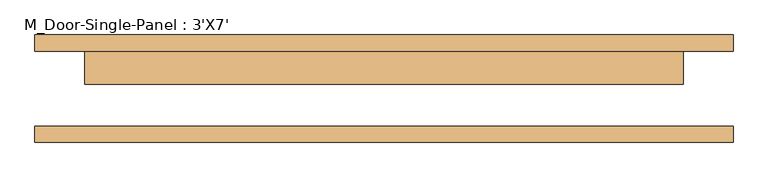
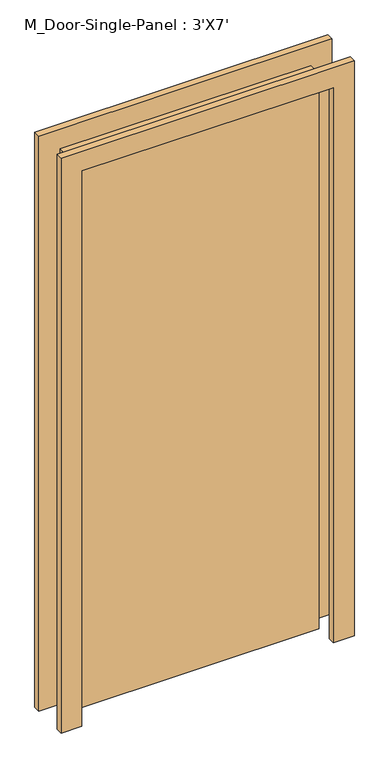
"""IFC4 building model written with IfcOpenShell, lengths in millimetres: door geometry, M_Door-Single-Panel : 3'X7'."""

from ifc_helpers import new_model, si_unit, frame, origin, origin_with_axes, place, context, project, spatial, polyline, outline, extrude, source, transform, mapped, element, save


def m_door_single_panel_3_x7_f8176753(model_context):
    return source(origin(), model_context, "Body", "SweptSolid", [
        extrude(outline(polyline([(457.2, 7.15), (-457.2, 7.15), (-457.2, 57.15), (457.2, 57.15), (457.2, 7.15)])), origin_with_axes(), (0.0, 0.0, 1.0), 2133.6),
        extrude(outline(polyline([(2209.8, 533.4), (2209.8, -533.4), (0.0, -533.4), (0.0, -457.2), (2133.6, -457.2), (2133.6, 457.2), (0.0, 457.2), (0.0, 533.4), (2209.8, 533.4)])), frame((0.0, -82.15, 0.0), z_axis=(0.0, 1.0, 0.0), x_axis=(0.0, 0.0, 1.0)), (0.0, 0.0, 1.0), 25.0),
        extrude(outline(polyline([(2209.8, -533.4), (0.0, -533.4), (0.0, -457.2), (2133.6, -457.2), (2133.6, 457.2), (0.0, 457.2), (0.0, 533.4), (2209.8, 533.4), (2209.8, -533.4)])), frame((0.0, 57.15, 0.0), z_axis=(0.0, 1.0, 0.0), x_axis=(0.0, 0.0, 1.0)), (0.0, 0.0, 1.0), 25.0),
    ])


if __name__ == "__main__":
    model = new_model("IFC4")
    model_context = context("Model", 3, world=origin())
    ifc_project = project(units=[si_unit("LENGTHUNIT", "METRE", prefix="MILLI")], contexts=[model_context])
    site = spatial("IfcSite", under=ifc_project)
    building = spatial("IfcBuilding", under=site)
    placement = place(None, origin())
    m_door_single_panel_3_x7_shape = m_door_single_panel_3_x7_f8176753(model_context)
    element("IfcDoor", 1, ObjectType="M_Door-Single-Panel : 3'X7'", at=placement, inside=building, context=model_context, shape_type="MappedRepresentation", body=[
        mapped(m_door_single_panel_3_x7_shape, transform((0.0, 0.0, 0.0), x_axis=(1.0, 0.0, 0.0), y_axis=(0.0, 1.0, 0.0), z_axis=(0.0, 0.0, 1.0))),
    ])
    save(model, "model.ifc")

# Revit data of these elements
# Type "M_Door-Single-Panel : 3'X7'"
#   Type Mark = "11"
#   Construction Type Id = "DOOR"
#   Assembly Code = "C1020300"
#   Analytic Construction = "Wooden"
#   Thickness = 0' - 1.9685"
#   Thermal Resistance (R) = 2.5876 (h·ft²·°F)/BTU
#   Swing Angle [instance default] = 90.00°
#   Heat Transfer Coefficient (U) = 0.3865 BTU/(h·ft²·°F)
#   Height = 7' - 0"
#   Trim Projection Ext = 0' - 0.98425"
#   Trim Projection Int = 0' - 0.98425"
#   Trim Width = 0' - 3.14961"
#   Width = 3' - 0"
#   Define Thermal Properties by = 1
#   Panel Material = Wood - Birch - Solid Stained Light Low Gloss
#   Trim Material = Paint - Sienna
#   Visual Light Transmittance = 0
#   Solar Heat Gain Coefficient = 0
#   Function = (empty or 0)
#   Wall Closure = (empty or 0)
# Element 1 (IfcDoor, "M_Door-Single-Panel : 3'X7'")
#   Materials on its faces: "Paint - Sienna", "Wood - Birch - Solid Stained Light Low Gloss"
# Materials
#   "Wood - Birch - Solid Stained Light Low Gloss": class "Wood", colour RGB 210 159 95, transparency 0, Cost = 0
#   "Paint - Sienna": colour RGB 118 70 51, transparency 0, Cost = 0
